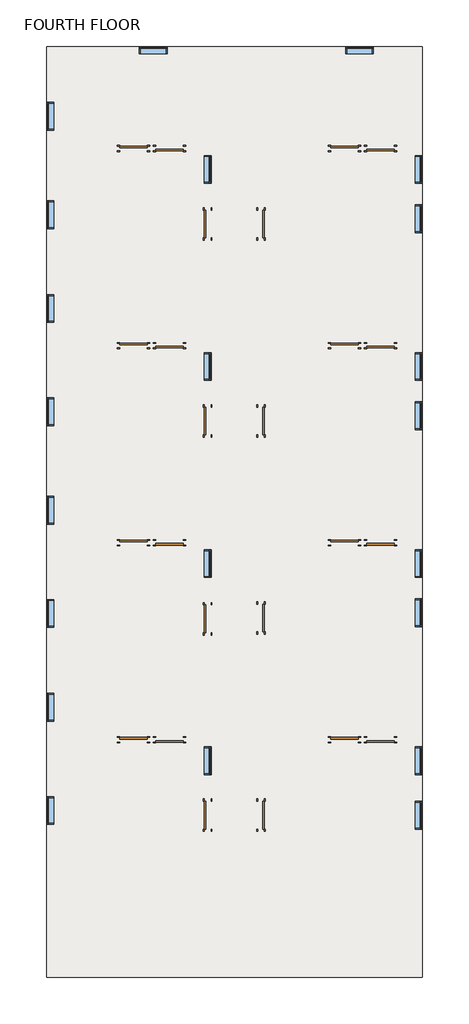
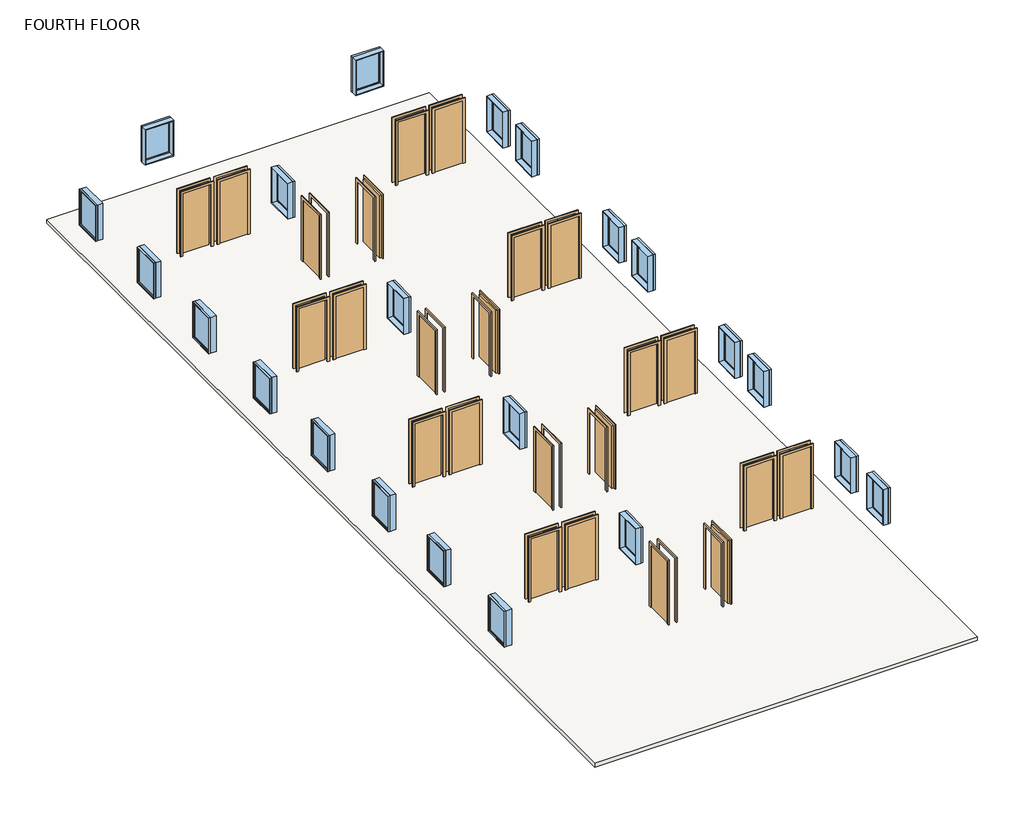
# One storey: 24 doors, 22 windows, 1 slab.
"""IFC4 building model written with IfcOpenShell, lengths in millimetres."""

from ifc_helpers import new_model, si_unit, frame, origin, place, context, project, spatial, polyline, outline, extrude, transform, mapped, element, save
from components import door_686f89d2, door_16372e1c, door_a90ba1ad, door_0ca8825f, window_c1f32544

model = new_model("IFC4")

# Units and contexts
model_context = context("Model", 3, world=origin())
ifc_project = project(units=[si_unit("LENGTHUNIT", "METRE", prefix="MILLI")], contexts=[model_context])

# Site, building, storey
site = spatial("IfcSite", under=ifc_project)
building = spatial("IfcBuilding", under=site)
storey = spatial("IfcBuildingStorey", under=building, Name="FOURTH FLOOR", Elevation=12801.6)

# Doors
placement = place(None, origin())
door_shape = door_686f89d2(model_context)
element("IfcDoor", 1, ObjectType="Single-Flush : 36\" x 84\"", at=placement, inside=storey, context=model_context, shape_type="MappedRepresentation", body=[
    mapped(door_shape, transform((-9863.5902461, 11952.2710592, 12801.6), x_axis=(-1.0, 0.0, 0.0), y_axis=(0.0, -1.0, 0.0), z_axis=(0.0, 0.0, 1.0))),
])
element("IfcDoor", 2, ObjectType="Single-Flush : 36\" x 84\"", at=placement, inside=storey, context=model_context, shape_type="MappedRepresentation", body=[
    mapped(door_shape, transform((-9863.5902461, 5475.2710592, 12801.6), x_axis=(-1.0, 0.0, 0.0), y_axis=(0.0, -1.0, 0.0), z_axis=(0.0, 0.0, 1.0))),
])
element("IfcDoor", 3, ObjectType="Single-Flush : 36\" x 84\"", at=placement, inside=storey, context=model_context, shape_type="MappedRepresentation", body=[
    mapped(door_shape, transform((-9863.5902461, -1001.7289408, 12801.6), x_axis=(-1.0, 0.0, 0.0), y_axis=(0.0, -1.0, 0.0), z_axis=(0.0, 0.0, 1.0))),
])
element("IfcDoor", 4, ObjectType="Single-Flush : 36\" x 84\"", at=placement, inside=storey, context=model_context, shape_type="MappedRepresentation", body=[
    mapped(door_shape, transform((-9863.5902461, -7478.7289408, 12801.6), x_axis=(-1.0, 0.0, 0.0), y_axis=(0.0, -1.0, 0.0), z_axis=(0.0, 0.0, 1.0))),
])
element("IfcDoor", 5, ObjectType="Single-Flush : 36\" x 84\"", at=placement, inside=storey, context=model_context, shape_type="MappedRepresentation", body=[
    mapped(door_shape, transform((-2929.3902461, -1001.7289408, 12801.6), x_axis=(-1.0, 0.0, 0.0), y_axis=(0.0, -1.0, 0.0), z_axis=(0.0, 0.0, 1.0))),
])
element("IfcDoor", 6, ObjectType="Single-Flush : 36\" x 84\"", at=placement, inside=storey, context=model_context, shape_type="MappedRepresentation", body=[
    mapped(door_shape, transform((-2929.3902461, 5475.2710592, 12801.6), x_axis=(-1.0, 0.0, 0.0), y_axis=(0.0, -1.0, 0.0), z_axis=(0.0, 0.0, 1.0))),
])
element("IfcDoor", 7, ObjectType="Single-Flush : 36\" x 84\"", at=placement, inside=storey, context=model_context, shape_type="MappedRepresentation", body=[
    mapped(door_shape, transform((-2929.3902461, 11952.2710592, 12801.6), x_axis=(-1.0, 0.0, 0.0), y_axis=(0.0, -1.0, 0.0), z_axis=(0.0, 0.0, 1.0))),
])
door_2_shape = door_16372e1c(model_context)
element("IfcDoor", 8, ObjectType="Single-Flush : 36\" x 84\"", at=placement, inside=storey, context=model_context, shape_type="MappedRepresentation", body=[
    mapped(door_2_shape, transform((-8682.4902461, 11952.2710592, 12801.6), x_axis=(-1.0, 0.0, 0.0), y_axis=(0.0, -1.0, 0.0), z_axis=(0.0, 0.0, 1.0))),
])
element("IfcDoor", 9, ObjectType="Single-Flush : 36\" x 84\"", at=placement, inside=storey, context=model_context, shape_type="MappedRepresentation", body=[
    mapped(door_2_shape, transform((-8682.4902461, 5475.2710592, 12801.6), x_axis=(-1.0, 0.0, 0.0), y_axis=(0.0, -1.0, 0.0), z_axis=(0.0, 0.0, 1.0))),
])
element("IfcDoor", 10, ObjectType="Single-Flush : 36\" x 84\"", at=placement, inside=storey, context=model_context, shape_type="MappedRepresentation", body=[
    mapped(door_2_shape, transform((-8682.4902461, -1001.7289408, 12801.6), x_axis=(-1.0, 0.0, 0.0), y_axis=(0.0, -1.0, 0.0), z_axis=(0.0, 0.0, 1.0))),
])
element("IfcDoor", 11, ObjectType="Single-Flush : 36\" x 84\"", at=placement, inside=storey, context=model_context, shape_type="MappedRepresentation", body=[
    mapped(door_2_shape, transform((-8682.4902461, -7478.7289408, 12801.6), x_axis=(-1.0, 0.0, 0.0), y_axis=(0.0, -1.0, 0.0), z_axis=(0.0, 0.0, 1.0))),
])
element("IfcDoor", 12, ObjectType="Single-Flush : 36\" x 84\"", at=placement, inside=storey, context=model_context, shape_type="MappedRepresentation", body=[
    mapped(door_2_shape, transform((-1748.2902461, -7478.7289408, 12801.6), x_axis=(-1.0, 0.0, 0.0), y_axis=(0.0, -1.0, 0.0), z_axis=(0.0, 0.0, 1.0))),
])
element("IfcDoor", 13, ObjectType="Single-Flush : 36\" x 84\"", at=placement, inside=storey, context=model_context, shape_type="MappedRepresentation", body=[
    mapped(door_2_shape, transform((-2929.3902461, -7478.7289408, 12801.6), x_axis=(1.0, 0.0, 0.0), y_axis=(0.0, 1.0, 0.0), z_axis=(0.0, 0.0, 1.0))),
])
element("IfcDoor", 14, ObjectType="Single-Flush : 36\" x 84\"", at=placement, inside=storey, context=model_context, shape_type="MappedRepresentation", body=[
    mapped(door_2_shape, transform((-1748.2902461, -1001.7289408, 12801.6), x_axis=(-1.0, 0.0, 0.0), y_axis=(0.0, -1.0, 0.0), z_axis=(0.0, 0.0, 1.0))),
])
element("IfcDoor", 15, ObjectType="Single-Flush : 36\" x 84\"", at=placement, inside=storey, context=model_context, shape_type="MappedRepresentation", body=[
    mapped(door_2_shape, transform((-1748.2902461, 5475.2710592, 12801.6), x_axis=(-1.0, 0.0, 0.0), y_axis=(0.0, -1.0, 0.0), z_axis=(0.0, 0.0, 1.0))),
])
element("IfcDoor", 16, ObjectType="Single-Flush : 36\" x 84\"", at=placement, inside=storey, context=model_context, shape_type="MappedRepresentation", body=[
    mapped(door_2_shape, transform((-1748.2902461, 11952.2710592, 12801.6), x_axis=(-1.0, 0.0, 0.0), y_axis=(0.0, -1.0, 0.0), z_axis=(0.0, 0.0, 1.0))),
])
door_3_shape = door_a90ba1ad(model_context)
element("IfcDoor", 17, ObjectType="Single-Flush : 36\" x 84\"", at=placement, inside=storey, context=model_context, shape_type="MappedRepresentation", body=[
    mapped(door_3_shape, transform((-7425.1902461, 9475.7710592, 12801.6), x_axis=(0.0, -1.0, 0.0), y_axis=(1.0, 0.0, 0.0), z_axis=(0.0, 0.0, 1.0))),
])
element("IfcDoor", 18, ObjectType="Single-Flush : 36\" x 84\"", at=placement, inside=storey, context=model_context, shape_type="MappedRepresentation", body=[
    mapped(door_3_shape, transform((-7425.1902461, 2998.7710592, 12801.6), x_axis=(0.0, -1.0, 0.0), y_axis=(1.0, 0.0, 0.0), z_axis=(0.0, 0.0, 1.0))),
])
element("IfcDoor", 19, ObjectType="Single-Flush : 36\" x 84\"", at=placement, inside=storey, context=model_context, shape_type="MappedRepresentation", body=[
    mapped(door_3_shape, transform((-7425.1902461, -3503.6289408, 12801.6), x_axis=(0.0, -1.0, 0.0), y_axis=(1.0, 0.0, 0.0), z_axis=(0.0, 0.0, 1.0))),
])
element("IfcDoor", 20, ObjectType="Single-Flush : 36\" x 84\"", at=placement, inside=storey, context=model_context, shape_type="MappedRepresentation", body=[
    mapped(door_3_shape, transform((-7425.1902461, -9955.2289408, 12801.6), x_axis=(0.0, -1.0, 0.0), y_axis=(1.0, 0.0, 0.0), z_axis=(0.0, 0.0, 1.0))),
])
door_4_shape = door_0ca8825f(model_context)
element("IfcDoor", 21, ObjectType="Single-Flush : 36\" x 84\"", at=placement, inside=storey, context=model_context, shape_type="MappedRepresentation", body=[
    mapped(door_4_shape, transform((-5672.5902461, 9475.7710592, 12801.6), x_axis=(0.0, -1.0, 0.0), y_axis=(1.0, 0.0, 0.0), z_axis=(0.0, 0.0, 1.0))),
])
element("IfcDoor", 22, ObjectType="Single-Flush : 36\" x 84\"", at=placement, inside=storey, context=model_context, shape_type="MappedRepresentation", body=[
    mapped(door_4_shape, transform((-5672.5902461, 2998.7710592, 12801.6), x_axis=(0.0, -1.0, 0.0), y_axis=(1.0, 0.0, 0.0), z_axis=(0.0, 0.0, 1.0))),
])
element("IfcDoor", 23, ObjectType="Single-Flush : 36\" x 84\"", at=placement, inside=storey, context=model_context, shape_type="MappedRepresentation", body=[
    mapped(door_4_shape, transform((-5672.5902461, -3478.2289408, 12801.6), x_axis=(0.0, -1.0, 0.0), y_axis=(1.0, 0.0, 0.0), z_axis=(0.0, 0.0, 1.0))),
])
element("IfcDoor", 24, ObjectType="Single-Flush : 36\" x 84\"", at=placement, inside=storey, context=model_context, shape_type="MappedRepresentation", body=[
    mapped(door_4_shape, transform((-5672.5902461, -9955.2289408, 12801.6), x_axis=(0.0, -1.0, 0.0), y_axis=(1.0, 0.0, 0.0), z_axis=(0.0, 0.0, 1.0))),
])

# Slab
element("IfcSlab", 25, ObjectType="Generic - 12\"", at=placement, inside=storey, context=model_context, shape_type="SweptSolid", body=[
    extrude(outline(polyline([(-376.6902461, 15305.0710592), (-376.6902461, -15289.2289408), (-12721.0902461, -15289.2289408), (-12721.0902461, 15305.0710592), (-376.6902461, 15305.0710592)])), frame((0.0, 0.0, 12674.6), z_axis=(0.0, 0.0, 1.0), x_axis=(1.0, 0.0, 0.0)), (0.0, 0.0, 1.0), 127.0),
])

# Windows
window_shape = window_c1f32544(model_context)
element("IfcWindow", 26, ObjectType="Fixed : 36\" x 48\"", at=placement, inside=storey, context=model_context, shape_type="MappedRepresentation", body=[
    mapped(window_shape, transform((-490.9902461, 11228.3710592, 12801.6), x_axis=(0.0, -1.0, 0.0), y_axis=(1.0, 0.0, 0.0), z_axis=(0.0, 0.0, 1.0))),
])
element("IfcWindow", 27, ObjectType="Fixed : 36\" x 48\"", at=placement, inside=storey, context=model_context, shape_type="MappedRepresentation", body=[
    mapped(window_shape, transform((-490.9902461, 9609.1210592, 12801.6), x_axis=(0.0, -1.0, 0.0), y_axis=(1.0, 0.0, 0.0), z_axis=(0.0, 0.0, 1.0))),
])
element("IfcWindow", 28, ObjectType="Fixed : 36\" x 48\"", at=placement, inside=storey, context=model_context, shape_type="MappedRepresentation", body=[
    mapped(window_shape, transform((-490.9902461, 4751.3710592, 12801.6), x_axis=(0.0, -1.0, 0.0), y_axis=(1.0, 0.0, 0.0), z_axis=(0.0, 0.0, 1.0))),
])
element("IfcWindow", 29, ObjectType="Fixed : 36\" x 48\"", at=placement, inside=storey, context=model_context, shape_type="MappedRepresentation", body=[
    mapped(window_shape, transform((-490.9902461, 3132.1210592, 12801.6), x_axis=(0.0, -1.0, 0.0), y_axis=(1.0, 0.0, 0.0), z_axis=(0.0, 0.0, 1.0))),
])
element("IfcWindow", 30, ObjectType="Fixed : 36\" x 48\"", at=placement, inside=storey, context=model_context, shape_type="MappedRepresentation", body=[
    mapped(window_shape, transform((-490.9902461, -1725.6289408, 12801.6), x_axis=(0.0, -1.0, 0.0), y_axis=(1.0, 0.0, 0.0), z_axis=(0.0, 0.0, 1.0))),
])
element("IfcWindow", 31, ObjectType="Fixed : 36\" x 48\"", at=placement, inside=storey, context=model_context, shape_type="MappedRepresentation", body=[
    mapped(window_shape, transform((-490.9902461, -3344.8789408, 12801.6), x_axis=(0.0, -1.0, 0.0), y_axis=(1.0, 0.0, 0.0), z_axis=(0.0, 0.0, 1.0))),
])
element("IfcWindow", 32, ObjectType="Fixed : 36\" x 48\"", at=placement, inside=storey, context=model_context, shape_type="MappedRepresentation", body=[
    mapped(window_shape, transform((-490.9902461, -8202.6289408, 12801.6), x_axis=(0.0, -1.0, 0.0), y_axis=(1.0, 0.0, 0.0), z_axis=(0.0, 0.0, 1.0))),
])
element("IfcWindow", 33, ObjectType="Fixed : 36\" x 48\"", at=placement, inside=storey, context=model_context, shape_type="MappedRepresentation", body=[
    mapped(window_shape, transform((-490.9902461, -9993.3289408, 12801.6), x_axis=(0.0, -1.0, 0.0), y_axis=(1.0, 0.0, 0.0), z_axis=(0.0, 0.0, 1.0))),
])
element("IfcWindow", 34, ObjectType="Fixed : 36\" x 48\"", at=placement, inside=storey, context=model_context, shape_type="MappedRepresentation", body=[
    mapped(window_shape, transform((-12606.7902461, -9764.7289408, 12801.6), x_axis=(0.0, 1.0, 0.0), y_axis=(-1.0, 0.0, 0.0), z_axis=(0.0, 0.0, 1.0))),
])
element("IfcWindow", 35, ObjectType="Fixed : 36\" x 48\"", at=placement, inside=storey, context=model_context, shape_type="MappedRepresentation", body=[
    mapped(window_shape, transform((-12606.7902461, -6373.8289408, 12801.6), x_axis=(0.0, 1.0, 0.0), y_axis=(-1.0, 0.0, 0.0), z_axis=(0.0, 0.0, 1.0))),
])
element("IfcWindow", 36, ObjectType="Fixed : 36\" x 48\"", at=placement, inside=storey, context=model_context, shape_type="MappedRepresentation", body=[
    mapped(window_shape, transform((-12606.7902461, -3287.7289408, 12801.6), x_axis=(0.0, 1.0, 0.0), y_axis=(-1.0, 0.0, 0.0), z_axis=(0.0, 0.0, 1.0))),
])
element("IfcWindow", 37, ObjectType="Fixed : 36\" x 48\"", at=placement, inside=storey, context=model_context, shape_type="MappedRepresentation", body=[
    mapped(window_shape, transform((-12606.7902461, 103.1710592, 12801.6), x_axis=(0.0, 1.0, 0.0), y_axis=(-1.0, 0.0, 0.0), z_axis=(0.0, 0.0, 1.0))),
])
element("IfcWindow", 38, ObjectType="Fixed : 36\" x 48\"", at=placement, inside=storey, context=model_context, shape_type="MappedRepresentation", body=[
    mapped(window_shape, transform((-12606.7902461, 3341.6710592, 12801.6), x_axis=(0.0, 1.0, 0.0), y_axis=(-1.0, 0.0, 0.0), z_axis=(0.0, 0.0, 1.0))),
])
element("IfcWindow", 39, ObjectType="Fixed : 36\" x 48\"", at=placement, inside=storey, context=model_context, shape_type="MappedRepresentation", body=[
    mapped(window_shape, transform((-12606.7902461, 6732.5710592, 12801.6), x_axis=(0.0, 1.0, 0.0), y_axis=(-1.0, 0.0, 0.0), z_axis=(0.0, 0.0, 1.0))),
])
element("IfcWindow", 40, ObjectType="Fixed : 36\" x 48\"", at=placement, inside=storey, context=model_context, shape_type="MappedRepresentation", body=[
    mapped(window_shape, transform((-12606.7902461, 9818.6710592, 12801.6), x_axis=(0.0, 1.0, 0.0), y_axis=(-1.0, 0.0, 0.0), z_axis=(0.0, 0.0, 1.0))),
])
element("IfcWindow", 41, ObjectType="Fixed : 36\" x 48\"", at=placement, inside=storey, context=model_context, shape_type="MappedRepresentation", body=[
    mapped(window_shape, transform((-12606.7902461, 13057.1710592, 12801.6), x_axis=(0.0, 1.0, 0.0), y_axis=(-1.0, 0.0, 0.0), z_axis=(0.0, 0.0, 1.0))),
])
element("IfcWindow", 42, ObjectType="Fixed : 36\" x 48\"", at=placement, inside=storey, context=model_context, shape_type="MappedRepresentation", body=[
    mapped(window_shape, transform((-9177.7902461, 15190.7710592, 12801.6), x_axis=(1.0, 0.0, 0.0), y_axis=(0.0, 1.0, 0.0), z_axis=(0.0, 0.0, 1.0))),
])
element("IfcWindow", 43, ObjectType="Fixed : 36\" x 48\"", at=placement, inside=storey, context=model_context, shape_type="MappedRepresentation", body=[
    mapped(window_shape, transform((-2395.9902461, 15190.7710592, 12801.6), x_axis=(1.0, 0.0, 0.0), y_axis=(0.0, 1.0, 0.0), z_axis=(0.0, 0.0, 1.0))),
])
element("IfcWindow", 44, ObjectType="Fixed : 36\" x 48\"", at=placement, inside=storey, context=model_context, shape_type="MappedRepresentation", body=[
    mapped(window_shape, transform((-7425.1902461, 4751.3710592, 12801.6), x_axis=(0.0, -1.0, 0.0), y_axis=(1.0, 0.0, 0.0), z_axis=(0.0, 0.0, 1.0))),
])
element("IfcWindow", 45, ObjectType="Fixed : 36\" x 48\"", at=placement, inside=storey, context=model_context, shape_type="MappedRepresentation", body=[
    mapped(window_shape, transform((-7425.1902461, -1725.6289408, 12801.6), x_axis=(0.0, -1.0, 0.0), y_axis=(1.0, 0.0, 0.0), z_axis=(0.0, 0.0, 1.0))),
])
element("IfcWindow", 46, ObjectType="Fixed : 36\" x 48\"", at=placement, inside=storey, context=model_context, shape_type="MappedRepresentation", body=[
    mapped(window_shape, transform((-7425.1902461, -8202.6289408, 12801.6), x_axis=(0.0, -1.0, 0.0), y_axis=(1.0, 0.0, 0.0), z_axis=(0.0, 0.0, 1.0))),
])
element("IfcWindow", 47, ObjectType="Fixed : 36\" x 48\"", at=placement, inside=storey, context=model_context, shape_type="MappedRepresentation", body=[
    mapped(window_shape, transform((-7425.1902461, 11228.3710592, 12801.6), x_axis=(0.0, -1.0, 0.0), y_axis=(1.0, 0.0, 0.0), z_axis=(0.0, 0.0, 1.0))),
])

save(model, "model.ifc")

# Revit data of these elements
# Type "Single-Flush : 36\" x 84\""
#   Type Mark = "1"
#   Construction Type Id = "MDOOR"
#   Assembly Code = "C1020"
#   Analytic Construction = "Metal"
#   Thickness = 0' - 2"
#   Heat Transfer Coefficient (U) = 0.651978 BTU/(h·ft²·°F)
#   Height = 7' - 0"
#   Trim Projection Ext = 0' - 1"
#   Trim Projection Int = 0' - 1"
#   Trim Width = 0' - 3"
#   Width = 3' - 0"
#   Define Thermal Properties by = 1
#   Door Material = Door - Panel
#   Frame Material = Door - Frame
#   Visual Light Transmittance = 0
#   Solar Heat Gain Coefficient = 0
#   Function = (empty or 0)
#   Wall Closure = (empty or 0)
# Type "Generic - 12\""
#   Assembly Code = "B1010"
#   Function = 0
#   Layers, outside or top first: 0' - 5" no material (function 1)
# Type "Fixed : 36\" x 48\""
#   Type Mark = "1"
#   Construction Type Id = "GSP4R"
#   Assembly Code = "B2020100"
#   Analytic Construction = "1/8 in Pilkington single glazing"
#   Visual Light Transmittance = 0.9
#   Solar Heat Gain Coefficient = 0.78
#   Heat Transfer Coefficient (U) = 0.6496 BTU/(h·ft²·°F)
#   Height = 4' - 0"
#   Default Sill Height = 3' - 0"
#   Width = 3' - 0"
#   Window Inset = 0' - 0 3/4"
#   Define Thermal Properties by = 1
#   Glass Pane Material = Glass
#   Sash Material = Sash
#   Wall Closure = (empty or 0)
# Elements 1, 2, 3, 4, 5, 6, 7, 8, 9, 10, 11, 12, 13, 14, 15, 16, 17, 18, 19, 20, 21, 22, 23, 24 (IfcDoor, "Single-Flush : 36\" x 84\"")
#   Phase Created = New Construction
#   Materials on its faces: "Door - Frame", "Door - Panel"
# Element 25 (IfcSlab, "Generic - 12\"")
#   Height Offset From Level = 0' - 0"
#   Phase Created = New Construction
#   Materials on its faces: "Default Floor"
# Element 26 (IfcWindow, "Fixed : 36\" x 48\"")
#   Mark = "93"
#   Phase Created = New Construction
#   Materials on its faces: "Sash", "Glass"
# Element 27 (IfcWindow, "Fixed : 36\" x 48\"")
#   Mark = "94"
#   Phase Created = New Construction
#   Materials on its faces: "Sash", "Glass"
# Element 28 (IfcWindow, "Fixed : 36\" x 48\"")
#   Mark = "95"
#   Phase Created = New Construction
#   Materials on its faces: "Sash", "Glass"
# Element 29 (IfcWindow, "Fixed : 36\" x 48\"")
#   Mark = "96"
#   Phase Created = New Construction
#   Materials on its faces: "Sash", "Glass"
# Element 30 (IfcWindow, "Fixed : 36\" x 48\"")
#   Mark = "97"
#   Phase Created = New Construction
#   Materials on its faces: "Sash", "Glass"
# Element 31 (IfcWindow, "Fixed : 36\" x 48\"")
#   Mark = "98"
#   Phase Created = New Construction
#   Materials on its faces: "Sash", "Glass"
# Element 32 (IfcWindow, "Fixed : 36\" x 48\"")
#   Mark = "99"
#   Phase Created = New Construction
#   Materials on its faces: "Sash", "Glass"
# Element 33 (IfcWindow, "Fixed : 36\" x 48\"")
#   Mark = "100"
#   Phase Created = New Construction
#   Materials on its faces: "Sash", "Glass"
# Element 34 (IfcWindow, "Fixed : 36\" x 48\"")
#   Mark = "101"
#   Phase Created = New Construction
#   Materials on its faces: "Sash", "Glass"
# Element 35 (IfcWindow, "Fixed : 36\" x 48\"")
#   Mark = "102"
#   Phase Created = New Construction
#   Materials on its faces: "Sash", "Glass"
# Element 36 (IfcWindow, "Fixed : 36\" x 48\"")
#   Mark = "103"
#   Phase Created = New Construction
#   Materials on its faces: "Sash", "Glass"
# Element 37 (IfcWindow, "Fixed : 36\" x 48\"")
#   Mark = "104"
#   Phase Created = New Construction
#   Materials on its faces: "Sash", "Glass"
# Element 38 (IfcWindow, "Fixed : 36\" x 48\"")
#   Mark = "105"
#   Phase Created = New Construction
#   Materials on its faces: "Sash", "Glass"
# Element 39 (IfcWindow, "Fixed : 36\" x 48\"")
#   Mark = "106"
#   Phase Created = New Construction
#   Materials on its faces: "Sash", "Glass"
# Element 40 (IfcWindow, "Fixed : 36\" x 48\"")
#   Mark = "107"
#   Phase Created = New Construction
#   Materials on its faces: "Sash", "Glass"
# Element 41 (IfcWindow, "Fixed : 36\" x 48\"")
#   Mark = "108"
#   Phase Created = New Construction
#   Materials on its faces: "Sash", "Glass"
# Element 42 (IfcWindow, "Fixed : 36\" x 48\"")
#   Mark = "109"
#   Phase Created = New Construction
#   Materials on its faces: "Sash", "Glass"
# Element 43 (IfcWindow, "Fixed : 36\" x 48\"")
#   Mark = "110"
#   Phase Created = New Construction
#   Materials on its faces: "Sash", "Glass"
# Element 44 (IfcWindow, "Fixed : 36\" x 48\"")
#   Mark = "111"
#   Phase Created = New Construction
#   Materials on its faces: "Sash", "Glass"
# Element 45 (IfcWindow, "Fixed : 36\" x 48\"")
#   Mark = "112"
#   Phase Created = New Construction
#   Materials on its faces: "Sash", "Glass"
# Element 46 (IfcWindow, "Fixed : 36\" x 48\"")
#   Mark = "113"
#   Phase Created = New Construction
#   Materials on its faces: "Sash", "Glass"
# Element 47 (IfcWindow, "Fixed : 36\" x 48\"")
#   Mark = "114"
#   Phase Created = New Construction
#   Materials on its faces: "Sash", "Glass"
# Materials
#   "Door - Panel": class "Wood", colour RGB 210 159 95, transparency 0
#   "Door - Frame": colour RGB 118 70 51, transparency 0
#   "Glass": class "Glass", colour RGB 0 128 192, transparency 0.75, Description = "Soda Lime Glass", Cost = 0
#   "Sash": class "Wood", colour RGB 224 178 126, transparency 0
#   "Default Floor": colour RGB 128 128 128, transparency 0
